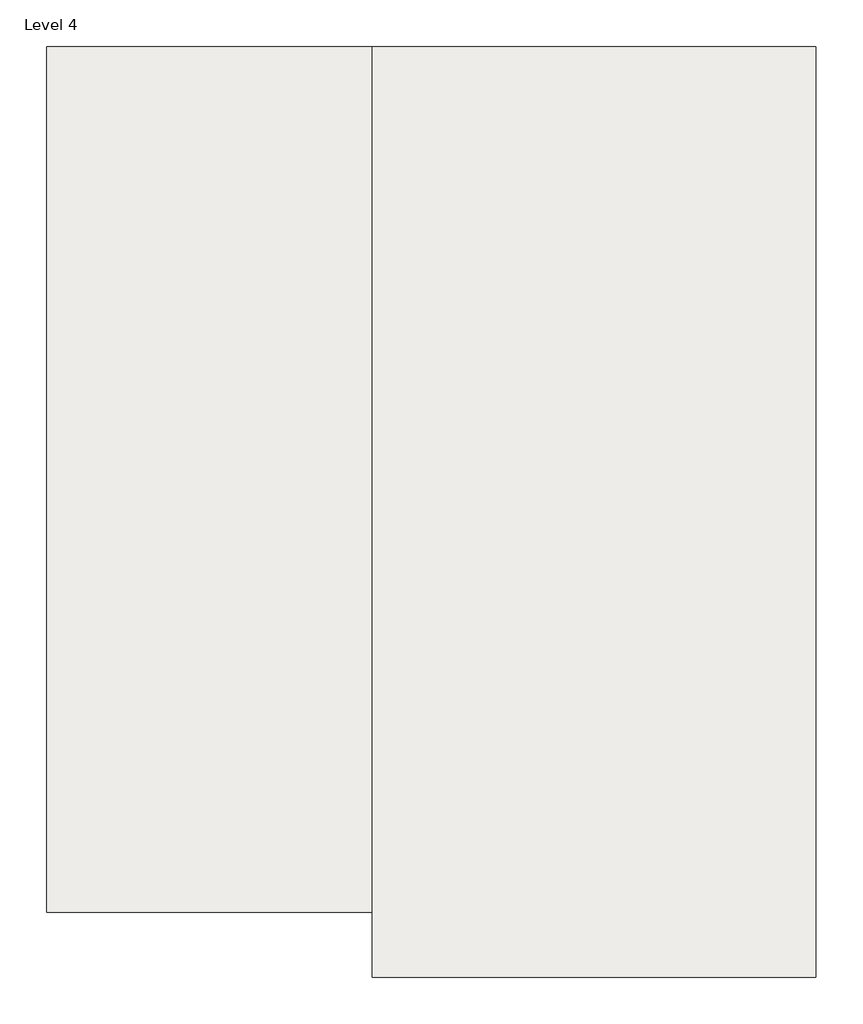
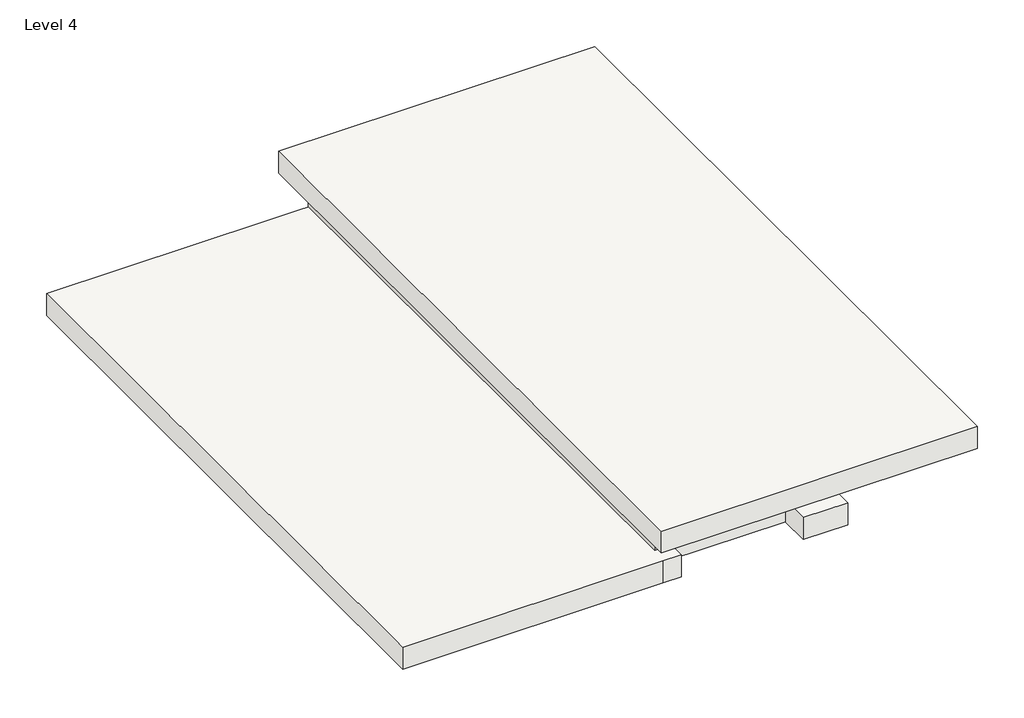
# One storey: 2 roofs, 2 walls.
"""IFC4 building model written with IfcOpenShell, lengths in millimetres."""

from ifc_helpers import new_model, si_unit, frame, origin, place, context, project, spatial, polyline, outline, extrude, faceted_brep, element, save

model = new_model("IFC4")

# Units and contexts
model_context = context("Model", 3, world=origin())
ifc_project = project(units=[si_unit("LENGTHUNIT", "METRE", prefix="MILLI")], contexts=[model_context])

# Site, building, storey
site = spatial("IfcSite", under=ifc_project)
building = spatial("IfcBuilding", under=site)
storey = spatial("IfcBuildingStorey", under=building, Name="Level 4", Elevation=10972.8)

# Roofs
placement = place(None, origin())
element("IfcRoof", 1, ObjectType="Generic - 12\"", at=placement, inside=storey, context=model_context, shape_type="SweptSolid", body=[
    extrude(outline(polyline([(-3753.7125658, 11743.1483979), (399.1874342, 11743.1483979), (399.1874342, 3030.9483979), (-3753.7125658, 3030.9483979), (-3753.7125658, 11743.1483979)])), frame((0.0, 0.0, 10972.8), z_axis=(0.0, 0.0, 1.0), x_axis=(1.0, 0.0, 0.0)), (0.0, 0.0, 1.0), 304.8),
])
element("IfcRoof", 2, ObjectType="Generic - 12\"", at=placement, inside=storey, context=model_context, shape_type="SweptSolid", body=[
    extrude(outline(polyline([(-6801.7125658, 11743.1483979), (-985.1125658, 11743.1483979), (-985.1125658, 4199.3483979), (-985.1125658, 3589.7483979), (-1567.4310441, 3589.7483979), (-1567.4310441, 3996.1483979), (-3142.2310441, 3996.1483979), (-3142.2310441, 3640.5483979), (-3385.4125658, 3640.5483979), (-6801.7125658, 3640.5483979), (-6801.7125658, 11743.1483979)])), frame((0.0, 0.0, 10058.4), z_axis=(0.0, 0.0, 1.0), x_axis=(1.0, 0.0, 0.0)), (0.0, 0.0, 1.0), 304.8),
])

# Walls
element("IfcWall", 3, ObjectType="Generic - 8\"", at=placement, inside=storey, context=model_context, shape_type="Brep", body=[
    faceted_brep([(-3156.8125658, 3869.1483979, 10363.2), (-3156.8125658, 11539.9483979, 10363.2), (-3156.8125658, 11743.1483979, 10363.2), (-3156.8125658, 11743.1483979, 10972.8), (-3156.8125658, 11539.9483979, 10972.8), (-3156.8125658, 3869.1483979, 10972.8), (-3360.0125658, 3869.1483979, 10363.2), (-3360.0125658, 3869.1483979, 10972.8), (-3360.0125658, 11743.1483979, 10972.8), (-3360.0125658, 11743.1483979, 10363.2)], [[[0, 1, 2, 3, 4, 5]], [[6, 7, 8, 9]], [[2, 1, 0, 6, 9]], [[5, 4, 3, 8, 7]], [[0, 5, 7, 6]], [[3, 2, 9, 8]]]),
])
element("IfcWall", 4, ObjectType="Generic - 8\"", at=placement, inside=storey, context=model_context, shape_type="SweptSolid", body=[
    extrude(outline(polyline([(-400.9125658, 11539.9483979), (-3156.8125658, 11539.9483979), (-3156.8125658, 11743.1483979), (-400.9125658, 11743.1483979), (-400.9125658, 11539.9483979)])), frame((0.0, 0.0, 10363.2), z_axis=(0.0, 0.0, 1.0), x_axis=(1.0, 0.0, 0.0)), (0.0, 0.0, 1.0), 609.6),
])

save(model, "model.ifc")

# Revit data of these elements
# Type "Generic - 12\""
#   Assembly Code = "B1020"
#   Layers, outside or top first: 1' - 0" no material (function 1)
# Type "Generic - 8\""
#   Assembly Code = "B2010"
#   Layers, outside or top first: 0' - 8" no material (function 1)
# Element 1 (IfcRoof, "Generic - 12\"")
#   built-in parameter 1001705 = 37 (stored number, unit not read)
#   built-in parameter 1001710 = 33615
#   Phase Created = New Construction
#   Materials on its faces: "Default Roof"
# Element 2 (IfcRoof, "Generic - 12\"")
#   built-in parameter 1001705 = 34 (stored number, unit not read)
#   built-in parameter 1001701 = -3 (stored number, unit not read)
#   built-in parameter 1001710 = 33615
#   Phase Created = New Construction
#   Materials on its faces: "Default Roof"
# Elements 3, 4 (IfcWall, "Generic - 8\"")
#   built-in parameter 1001111 = -2' - 0"
#   Top Offset = 0' - 0"
#   Base Offset = -2' - 0"
#   Unconnected Height = 2' - 0"
#   wall height = 2' - 0"
#   Phase Created = New Construction
#   Base Constraint = Level 4
#   Materials on its faces: "Default Wall"
# Materials
#   "Default Roof": colour RGB 88 101 114, transparency 0
#   "Default Wall": colour RGB 128 128 128, transparency 0
